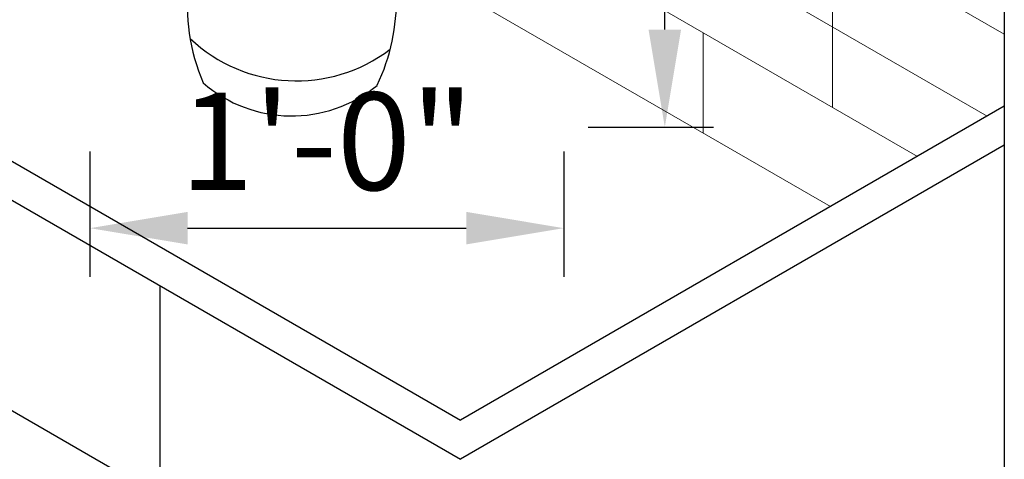
# Model space of a CAD drawing. Units: inches. Extents: x 5770 to 11891, y 3254 to 6808.
# Tile 9 of 15: x 6048 to 6073, y 3403 to 3414. Entities that reach past the tile are written whole.
import ezdxf

# ---------------------------------------------------------------- set-up
doc = ezdxf.new("R2010")
doc.units = ezdxf.units.IN
for name, color, linetype, lineweight in [('A-ANNO-DIMS', 2, 'Continuous', 18), ('A-DOOR', 4, 'Continuous', 25), ('A-FURN', 8, 'Continuous', 25), ('A-WALL-PATT', 8, 'Continuous', 13)]:
    doc.layers.add(name, color=color, linetype=linetype, lineweight=lineweight)
doc.styles.get("Standard").update_dxf_attribs({"font": 'arial.ttf'})
doc.dimstyles.new('ISO-25', dxfattribs={"dimtxt": 2.5, "dimasz": 2.5, "dimexe": 1.25, "dimexo": 0.625, "dimtad": 1, "dimdec": 0, "dimlunit": 3, "dimtxsty": 'Standard', "dimcen": 2.5, "dimadec": 0, "dimazin": 0, "dimtfac": 1, "dimtdec": 0, "dimtmove": 0, "dimatfit": 3, "dimfxl": 1, "dimarcsym": 0})

# ---------------------------------------------------------------- blocks, each defined once
blk = doc.blocks.new('POT TREE')
for centre, radius, start, end in [((6057.241, 3414.341), 4.914, 142.3065, 203.4115), ((6052.61, 3414.509), 5.072, 334.4796, 28.1737), ((6055.12, 3416.4), 3.962, 226.5306, 307.3215), ((6054.997, 3414.987), 3.448, 228.9077, 309.4208)]:
    blk.add_arc(centre, radius, start, end)
blk.add_ellipse((6055.216, 3417.125), major_axis=(-1.864, 0.221), ratio=0.431649, start_param=4.964377, end_param=10.722247)
for points, knots in [([(6056.099, 3428.486), (6056.067, 3428.368), (6056.02, 3428.192), (6055.948, 3427.91), (6056.053, 3427.786), (6056.115, 3427.713)], [0, 0, 0, 0, 0.3734405, 0.5554394, 0.8239698, 0.8239698, 0.8239698, 0.8239698]), ([(6056.207, 3427.847), (6056.213, 3427.924), (6056.224, 3428.053), (6056.232, 3428.215), (6056.298, 3428.293), (6056.297, 3428.355), (6056.343, 3428.437), (6056.403, 3428.481), (6056.451, 3428.516)], [0, 0, 0, 0, 0.2339594, 0.3926456, 0.4649395, 0.5251746, 0.5691994, 0.7434006, 0.7434006, 0.7434006, 0.7434006]), ([(6055.216, 3417.125), (6055.336, 3418.48), (6055.487, 3420.181), (6056.331, 3422.342), (6055.715, 3423.715), (6056.354, 3425.55), (6055.582, 3427.539), (6056.504, 3428.093), (6056.597, 3428.149)], [0, 0, 0, 0, 4.080433, 5.124412, 6.755782, 8.14589, 10.974647, 11.292118, 11.292118, 11.292118, 11.292118]), ([(6056, 3427.411), (6055.979, 3427.477), (6055.946, 3427.582), (6055.946, 3427.752), (6055.806, 3427.869), (6055.784, 3428.034), (6055.784, 3428.159), (6055.766, 3428.202), (6055.759, 3428.218)], [0, 0, 0, 0, 0.2083526, 0.33199, 0.4828354, 0.7148467, 0.8018251, 0.8541407, 0.8541407, 0.8541407, 0.8541407]), ([(6056.371, 3428.002), (6056.422, 3428.039), (6056.532, 3428.118), (6056.727, 3428.199), (6056.886, 3428.139), (6056.964, 3428.199), (6056.961, 3428.223), (6056.96, 3428.232)], [0, 0, 0, 0, 0.1895566, 0.4093046, 0.6024508, 0.6414497, 0.6690189, 0.6690189, 0.6690189, 0.6690189]), ([(6055.967, 3426.585), (6055.915, 3426.698), (6055.838, 3426.866), (6055.755, 3427.096), (6055.662, 3427.248), (6055.479, 3427.316), (6055.344, 3427.566), (6055.436, 3427.759), (6055.492, 3427.874)], [0, 0, 0, 0, 0.371816, 0.552306, 0.74044, 0.877889, 1.120726, 1.482251, 1.482251, 1.482251, 1.482251]), ([(6056.064, 3427.611), (6056.145, 3427.655), (6056.269, 3427.724), (6056.427, 3427.889), (6056.588, 3427.869), (6056.72, 3427.903), (6056.741, 3427.953), (6056.749, 3427.972)], [0, 0, 0, 0, 0.2777951, 0.4294687, 0.6442569, 0.739735, 0.8005553, 0.8005553, 0.8005553, 0.8005553]), ([(6059.539, 3427.305), (6059.549, 3427.361), (6059.566, 3427.456), (6059.622, 3427.589), (6059.57, 3427.693), (6059.584, 3427.781), (6059.582, 3427.83), (6059.582, 3427.851)], [0, 0, 0, 0, 0.170284, 0.2915753, 0.4095788, 0.4920381, 0.5552227, 0.5552227, 0.5552227, 0.5552227]), ([(6055.746, 3427.727), (6055.745, 3427.704), (6055.742, 3427.656), (6055.802, 3427.595), (6055.813, 3427.51), (6055.793, 3427.397), (6055.923, 3427.324), (6055.949, 3427.228), (6055.963, 3427.179)], [0, 0, 0, 0, 0.0663677, 0.1385674, 0.2396579, 0.315315, 0.459478, 0.6088633, 0.6088633, 0.6088633, 0.6088633]), ([(6055.99, 3427.367), (6056.038, 3427.373), (6056.112, 3427.383), (6056.172, 3427.461), (6056.237, 3427.541), (6056.366, 3427.57), (6056.481, 3427.602), (6056.575, 3427.618), (6056.602, 3427.667), (6056.64, 3427.68), (6056.661, 3427.712), (6056.683, 3427.71), (6056.69, 3427.709)], [0, 0, 0, 0, 0.1365482, 0.2128619, 0.286554, 0.4402885, 0.5819688, 0.663825, 0.70336, 0.7384662, 0.7808805, 0.8013382, 0.8013382, 0.8013382, 0.8013382]), ([(6059.29, 3426.939), (6059.259, 3427.006), (6059.196, 3427.136), (6059.318, 3427.315), (6059.332, 3427.522), (6059.269, 3427.641), (6059.235, 3427.705)], [0, 0, 0, 0, 0.2050478, 0.4040971, 0.5914015, 0.8021175, 0.8021175, 0.8021175, 0.8021175]), ([(6059.29, 3426.939), (6059.343, 3427.011), (6059.426, 3427.125), (6059.515, 3427.313), (6059.674, 3427.364), (6059.891, 3427.379), (6059.816, 3427.58), (6059.884, 3427.567), (6059.904, 3427.563)], [0, 0, 0, 0, 0.2714027, 0.4305119, 0.5814667, 0.7785807, 0.9004742, 0.951926, 0.951926, 0.951926, 0.951926]), ([(6056.605, 3427.524), (6056.509, 3427.444), (6056.38, 3427.336), (6056.327, 3427.13), (6056.226, 3427.052), (6056.128, 3427.019), (6056.036, 3426.975), (6056.021, 3426.89), (6055.939, 3426.905), (6055.963, 3426.892), (6055.973, 3426.886)], [0, 0, 0, 0, 0.3596279, 0.4887998, 0.612961, 0.7210682, 0.8063572, 0.9000005, 0.9307269, 0.9560982, 0.9560982, 0.9560982, 0.9560982]), ([(6055.977, 3426.474), (6055.99, 3426.502), (6056.028, 3426.582), (6056.121, 3426.639), (6056.2, 3426.712), (6056.242, 3426.835), (6056.362, 3426.959), (6056.525, 3427.032), (6056.66, 3427.104), (6056.792, 3427.159), (6056.821, 3427.278), (6056.814, 3427.378), (6056.873, 3427.411), (6056.899, 3427.426)], [0, 0, 0, 0, 0.092214, 0.262657, 0.315664, 0.410651, 0.642816, 0.809137, 0.941877, 1.112577, 1.190652, 1.298465, 1.380948, 1.380948, 1.380948, 1.380948]), ([(6056.095, 3422.726), (6056.606, 3423.324), (6057.847, 3424.774), (6058.906, 3426.363), (6059.529, 3427.297)], [0, 0, 0, 0, 2.356363, 5.722003, 5.722003, 5.722003, 5.722003]), ([(6056.056, 3425.848), (6056.006, 3425.989), (6055.924, 3426.218), (6055.821, 3426.517), (6055.761, 3426.712), (6055.708, 3426.876), (6055.625, 3426.962), (6055.572, 3427.054), (6055.493, 3427.115), (6055.42, 3427.147), (6055.376, 3427.166)], [0, 0, 0, 0, 0.450624, 0.730149, 0.944944, 1.068285, 1.240151, 1.294175, 1.386296, 1.531529, 1.531529, 1.531529, 1.531529]), ([(6058.831, 3426.258), (6058.841, 3426.314), (6058.865, 3426.442), (6058.859, 3426.622), (6058.864, 3426.782), (6058.891, 3426.906), (6058.89, 3427.037), (6058.917, 3427.145), (6058.938, 3427.235), (6058.962, 3427.266), (6058.975, 3427.282)], [0, 0, 0, 0, 0.170516, 0.389854, 0.537702, 0.648645, 0.771235, 0.925907, 0.983276, 1.044113, 1.044113, 1.044113, 1.044113]), ([(6059.29, 3426.939), (6059.328, 3426.955), (6059.413, 3426.99), (6059.547, 3427.012), (6059.733, 3427.027), (6059.904, 3427.081), (6060.076, 3427.185), (6060.184, 3427.182), (6060.249, 3427.18)], [0, 0, 0, 0, 0.1235803, 0.275185, 0.4036544, 0.6827396, 0.8054315, 0.9964413, 0.9964413, 0.9964413, 0.9964413]), ([(6056.054, 3424.972), (6055.977, 3425.109), (6055.832, 3425.363), (6055.757, 3425.794), (6055.716, 3426.157), (6055.592, 3426.405), (6055.526, 3426.622), (6055.441, 3426.739), (6055.385, 3426.816)], [0, 0, 0, 0, 0.467532, 0.868461, 1.30425, 1.550258, 1.694478, 1.979135, 1.979135, 1.979135, 1.979135]), ([(6056.377, 3426.818), (6056.352, 3426.755), (6056.308, 3426.64), (6056.245, 3426.496), (6056.206, 3426.387), (6056.142, 3426.323), (6056.096, 3426.241), (6056.077, 3426.145), (6056.033, 3426.102), (6056.017, 3426.086)], [0, 0, 0, 0, 0.2037441, 0.3695408, 0.4757745, 0.5419956, 0.6389372, 0.7550592, 0.8219377, 0.8219377, 0.8219377, 0.8219377]), ([(6056.056, 3425.848), (6056.123, 3425.96), (6056.303, 3426.262), (6056.779, 3426.349), (6056.935, 3426.684), (6056.925, 3426.814), (6056.92, 3426.871)], [0, 0, 0, 0, 0.381595, 1.02877, 1.247836, 1.417617, 1.417617, 1.417617, 1.417617]), ([(6058.261, 3425.438), (6058.291, 3425.526), (6058.343, 3425.679), (6058.339, 3425.9), (6058.37, 3426.087), (6058.319, 3426.305), (6058.353, 3426.513), (6058.32, 3426.678), (6058.317, 3426.794), (6058.344, 3426.858), (6058.363, 3426.902)], [0, 0, 0, 0, 0.275722, 0.478551, 0.660336, 0.838715, 1.138147, 1.278337, 1.3416, 1.482993, 1.482993, 1.482993, 1.482993]), ([(6058.563, 3425.867), (6058.56, 3426.061), (6058.555, 3426.39), (6058.4, 3426.795), (6058.513, 3426.977), (6058.549, 3427.032), (6058.551, 3427.035)], [0, 0, 0, 0, 0.586596, 0.998805, 1.183674, 1.195699, 1.195699, 1.195699, 1.195699]), ([(6058.962, 3426.451), (6059.049, 3426.488), (6059.206, 3426.554), (6059.435, 3426.627), (6059.634, 3426.652), (6059.81, 3426.698), (6059.948, 3426.696), (6060.018, 3426.762), (6060.066, 3426.814), (6060.121, 3426.838), (6060.156, 3426.854)], [0, 0, 0, 0, 0.283693, 0.509561, 0.721223, 0.878225, 1.064501, 1.097071, 1.163997, 1.27537, 1.27537, 1.27537, 1.27537]), ([(6059.16, 3426.744), (6059.203, 3426.742), (6059.314, 3426.736), (6059.465, 3426.81), (6059.623, 3426.872), (6059.755, 3426.911), (6059.886, 3426.903), (6059.993, 3426.931), (6060.073, 3426.99), (6060.123, 3427.004), (6060.148, 3427.011)], [0, 0, 0, 0, 0.127889, 0.331448, 0.488133, 0.640962, 0.738356, 0.878783, 0.95994, 1.034357, 1.034357, 1.034357, 1.034357]), ([(6055.951, 3424.314), (6055.922, 3424.36), (6055.81, 3424.54), (6055.651, 3424.735), (6055.521, 3424.997), (6055.443, 3425.215), (6055.337, 3425.488), (6054.988, 3425.625), (6055.168, 3425.925), (6055.049, 3426.109), (6054.991, 3426.355), (6054.968, 3426.555), (6054.951, 3426.702)], [0, 0, 0, 0, 0.163711, 0.635891, 0.747378, 1.038356, 1.335228, 1.608013, 1.929766, 2.083186, 2.238732, 2.684923, 2.684923, 2.684923, 2.684923]), ([(6057.656, 3424.618), (6057.652, 3424.844), (6057.647, 3425.111), (6057.61, 3425.475), (6057.704, 3425.744), (6057.631, 3426.115), (6057.55, 3426.461), (6057.608, 3426.662), (6057.627, 3426.731)], [0, 0, 0, 0, 0.681083, 0.80233, 1.088716, 1.507668, 1.913958, 2.127718, 2.127718, 2.127718, 2.127718]), ([(6057.812, 3424.824), (6057.859, 3424.939), (6057.966, 3425.201), (6057.98, 3425.575), (6057.986, 3425.877), (6058.063, 3426.137), (6057.992, 3426.354), (6057.93, 3426.581), (6057.997, 3426.635), (6058.014, 3426.65)], [0, 0, 0, 0, 0.369909, 0.844557, 1.104784, 1.280935, 1.632037, 1.811788, 1.877667, 1.877667, 1.877667, 1.877667]), ([(6056.072, 3425.293), (6056.133, 3425.505), (6056.266, 3425.967), (6056.936, 3426.129), (6056.94, 3426.432), (6056.94, 3426.477)], [0, 0, 0, 0, 0.63578, 1.387331, 1.51754, 1.51754, 1.51754, 1.51754]), ([(6057.341, 3423.955), (6057.366, 3424.231), (6057.406, 3424.685), (6057.283, 3425.234), (6057.35, 3425.634), (6057.475, 3425.987), (6057.255, 3426.274), (6057.321, 3426.442), (6057.341, 3426.491)], [0, 0, 0, 0, 0.827857, 1.361014, 1.650618, 2.046768, 2.412651, 2.567148, 2.567148, 2.567148, 2.567148]), ([(6058.777, 3426.179), (6058.935, 3426.238), (6059.178, 3426.33), (6059.474, 3426.418), (6059.645, 3426.392), (6059.742, 3426.437), (6059.823, 3426.499), (6059.909, 3426.479), (6059.995, 3426.5), (6060.058, 3426.496), (6060.091, 3426.519), (6060.093, 3426.521)], [0, 0, 0, 0, 0.507912, 0.783706, 0.910821, 1.010253, 1.096153, 1.201661, 1.253677, 1.364003, 1.37374, 1.37374, 1.37374, 1.37374]), ([(6056.038, 3424.843), (6056.072, 3424.898), (6056.124, 3424.984), (6056.15, 3425.124), (6056.224, 3425.253), (6056.367, 3425.285), (6056.418, 3425.409), (6056.447, 3425.536), (6056.633, 3425.585), (6056.578, 3425.765), (6056.728, 3425.791), (6056.822, 3425.814), (6056.921, 3425.958), (6057.035, 3426.009), (6057.139, 3426.056)], [0, 0, 0, 0, 0.192002, 0.297038, 0.424323, 0.617299, 0.671515, 0.818658, 0.985168, 1.116162, 1.215874, 1.36714, 1.40004, 1.729093, 1.729093, 1.729093, 1.729093]), ([(6058.635, 3425.972), (6058.738, 3426.004), (6058.893, 3426.052), (6059.061, 3426.159), (6059.218, 3426.171), (6059.334, 3426.132), (6059.411, 3426.181), (6059.424, 3426.213), (6059.433, 3426.237), (6059.438, 3426.25)], [0, 0, 0, 0, 0.3205478, 0.4875046, 0.5825134, 0.7880727, 0.8113343, 0.8451959, 0.8888695, 0.8888695, 0.8888695, 0.8888695]), ([(6055.908, 3423.774), (6055.633, 3423.935), (6055.268, 3424.15), (6055.37, 3424.761), (6054.903, 3424.997), (6054.405, 3425.105), (6054.23, 3425.467), (6053.986, 3425.639), (6053.974, 3425.758), (6053.967, 3425.819)], [0, 0, 0, 0, 0.828493, 1.099501, 1.668133, 2.09953, 2.614238, 2.775429, 2.952527, 2.952527, 2.952527, 2.952527]), ([(6055.474, 3425.905), (6055.51, 3425.799), (6055.556, 3425.669), (6055.622, 3425.499), (6055.623, 3425.305), (6055.834, 3425.19), (6055.818, 3425.005), (6055.912, 3424.948), (6055.91, 3424.824), (6055.955, 3424.719), (6055.995, 3424.675), (6056.01, 3424.659)], [0, 0, 0, 0, 0.336378, 0.413394, 0.545538, 0.892702, 0.982578, 1.034981, 1.194475, 1.310114, 1.373927, 1.373927, 1.373927, 1.373927]), ([(6058.421, 3425.664), (6058.505, 3425.707), (6058.644, 3425.779), (6058.864, 3425.834), (6059.06, 3425.877), (6059.217, 3425.861), (6059.319, 3425.896), (6059.371, 3425.9), (6059.397, 3425.925), (6059.403, 3425.931)], [0, 0, 0, 0, 0.283751, 0.46616, 0.680012, 0.883292, 0.92268, 1.004792, 1.029716, 1.029716, 1.029716, 1.029716]), ([(6055.951, 3424.314), (6055.971, 3424.342), (6056.04, 3424.439), (6056.158, 3424.572), (6056.282, 3424.757), (6056.522, 3424.974), (6056.461, 3425.359), (6056.847, 3425.665), (6057.142, 3425.719), (6057.374, 3425.762)], [0, 0, 0, 0, 0.103537, 0.354957, 0.533042, 0.771117, 1.289622, 1.481323, 2.177692, 2.177692, 2.177692, 2.177692]), ([(6058.261, 3425.438), (6058.37, 3425.457), (6058.551, 3425.488), (6058.776, 3425.584), (6058.921, 3425.67), (6059.047, 3425.695), (6059.147, 3425.687), (6059.211, 3425.696), (6059.244, 3425.701)], [0, 0, 0, 0, 0.330364, 0.547312, 0.729955, 0.831797, 0.929171, 1.027126, 1.027126, 1.027126, 1.027126]), ([(6055.918, 3424.061), (6055.807, 3424.119), (6055.605, 3424.225), (6055.669, 3424.572), (6055.437, 3424.761), (6055.344, 3425.012), (6055.093, 3425.129), (6054.941, 3425.333), (6054.69, 3425.32), (6054.659, 3425.414), (6054.651, 3425.437)], [0, 0, 0, 0, 0.336493, 0.612709, 0.889575, 1.168065, 1.376144, 1.687858, 1.898629, 1.969205, 1.969205, 1.969205, 1.969205]), ([(6058.016, 3425.1), (6058.09, 3425.123), (6058.24, 3425.171), (6058.377, 3425.249), (6058.448, 3425.288)], [0, 0, 0, 0, 0.2298962, 0.4721725, 0.4721725, 0.4721725, 0.4721725]), ([(6058.448, 3425.288), (6058.521, 3425.33), (6058.626, 3425.39), (6058.771, 3425.413), (6058.839, 3425.441), (6058.89, 3425.468), (6059.001, 3425.522), (6059.117, 3425.5), (6059.209, 3425.483)], [0, 0, 0, 0, 0.2475713, 0.3610151, 0.4350864, 0.4658518, 0.5335827, 0.8019321, 0.8019321, 0.8019321, 0.8019321]), ([(6057.656, 3424.618), (6057.702, 3424.649), (6057.811, 3424.723), (6057.967, 3424.784), (6058.092, 3424.912), (6058.24, 3424.946), (6058.406, 3424.93), (6058.532, 3424.97), (6058.635, 3424.985), (6058.698, 3425.029), (6058.74, 3425.056), (6058.818, 3425.086), (6058.86, 3425.114), (6058.898, 3425.14)], [0, 0, 0, 0, 0.169056, 0.394003, 0.492513, 0.697087, 0.817485, 0.993544, 1.088828, 1.12295, 1.222592, 1.236685, 1.373008, 1.373008, 1.373008, 1.373008]), ([(6052.095, 3424.128), (6051.893, 3424.174), (6051.588, 3424.244), (6051.432, 3424.772), (6050.96, 3424.716), (6050.677, 3424.834), (6050.499, 3424.886), (6050.399, 3424.881), (6050.277, 3424.893), (6050.323, 3424.931), (6050.355, 3424.957)], [0, 0, 0, 0, 0.567769, 0.855404, 1.45352, 1.680633, 1.805502, 1.990259, 2.022667, 2.10403, 2.10403, 2.10403, 2.10403]), ([(6052.343, 3424.042), (6052.218, 3424.175), (6052.017, 3424.389), (6051.803, 3424.65), (6051.728, 3424.895), (6051.471, 3424.824), (6051.572, 3425.006), (6051.486, 3424.99), (6051.442, 3424.981)], [0, 0, 0, 0, 0.542059, 0.875538, 1.040909, 1.212562, 1.305796, 1.401779, 1.401779, 1.401779, 1.401779]), ([(6055.908, 3423.774), (6056.079, 3423.881), (6056.273, 3424.004), (6056.294, 3424.296), (6056.442, 3424.382), (6056.436, 3424.57), (6056.566, 3424.599), (6056.652, 3424.629), (6056.706, 3424.683), (6056.749, 3424.715), (6056.785, 3424.758), (6056.813, 3424.79), (6056.828, 3424.806)], [0, 0, 0, 0, 0.542154, 0.617715, 0.844166, 0.985871, 1.075503, 1.203366, 1.260039, 1.30062, 1.363236, 1.427954, 1.427954, 1.427954, 1.427954]), ([(6057.262, 3424.117), (6057.321, 3424.22), (6057.45, 3424.44), (6057.801, 3424.465), (6057.98, 3424.628), (6058.071, 3424.73), (6058.139, 3424.775), (6058.206, 3424.814), (6058.293, 3424.816), (6058.392, 3424.838), (6058.585, 3424.884), (6058.731, 3424.952), (6058.845, 3425.005)], [0, 0, 0, 0, 0.337635, 0.723781, 0.946218, 1.049759, 1.130989, 1.190526, 1.278087, 1.386469, 1.496256, 1.869563, 1.869563, 1.869563, 1.869563]), ([(6053.102, 3423.341), (6052.97, 3423.509), (6052.8, 3423.727), (6052.762, 3424.081), (6052.701, 3424.27), (6052.615, 3424.453), (6052.462, 3424.594), (6052.282, 3424.626), (6052.055, 3424.59), (6052.073, 3424.693), (6052.08, 3424.733)], [0, 0, 0, 0, 0.618637, 0.799298, 1.058478, 1.209073, 1.406969, 1.64005, 1.800082, 1.901705, 1.901705, 1.901705, 1.901705]), ([(6059.336, 3423.893), (6059.408, 3424.012), (6059.539, 3424.232), (6059.834, 3424.307), (6059.954, 3424.433), (6059.99, 3424.55), (6060.142, 3424.55), (6060.219, 3424.694), (6060.331, 3424.733), (6060.401, 3424.761), (6060.419, 3424.769)], [0, 0, 0, 0, 0.400751, 0.736445, 0.858272, 0.903351, 1.088652, 1.199604, 1.364928, 1.425221, 1.425221, 1.425221, 1.425221]), ([(6060.005, 3424.184), (6060.12, 3424.224), (6060.289, 3424.284), (6060.491, 3424.373), (6060.647, 3424.398), (6060.679, 3424.537), (6060.828, 3424.549), (6060.995, 3424.593), (6061.2, 3424.559), (6061.253, 3424.642), (6061.255, 3424.646)], [0, 0, 0, 0, 0.362377, 0.533627, 0.680662, 0.781131, 0.894461, 1.071848, 1.350792, 1.364242, 1.364242, 1.364242, 1.364242]), ([(6051.253, 3424.176), (6051.125, 3424.167), (6050.939, 3424.154), (6050.737, 3424.369), (6050.418, 3424.319), (6050.137, 3424.329), (6049.924, 3424.328), (6049.85, 3424.328), (6049.829, 3424.328)], [0, 0, 0, 0, 0.359068, 0.523067, 0.822385, 1.235556, 1.394449, 1.458006, 1.458006, 1.458006, 1.458006]), ([(6055.646, 3420.285), (6054.953, 3420.935), (6053.781, 3422.034), (6052.605, 3424.433), (6051.084, 3424.175), (6050.302, 3424.043)], [0, 0, 0, 0, 2.90941, 4.916012, 7.044236, 7.044236, 7.044236, 7.044236]), ([(6053.304, 3423.041), (6053.281, 3423.107), (6053.242, 3423.221), (6053.213, 3423.38), (6053.212, 3423.562), (6053.093, 3423.731), (6053.031, 3423.964), (6053.134, 3424.1), (6053.132, 3424.22), (6053.101, 3424.267), (6053.085, 3424.294)], [0, 0, 0, 0, 0.211774, 0.357994, 0.485633, 0.747154, 0.967772, 1.145664, 1.219006, 1.311906, 1.311906, 1.311906, 1.311906]), ([(6054.095, 3421.885), (6053.944, 3422.23), (6053.77, 3422.627), (6053.839, 3423.155), (6053.889, 3423.378), (6053.801, 3423.541), (6053.791, 3423.682), (6053.725, 3423.875), (6053.744, 3424.161), (6053.726, 3424.363), (6053.717, 3424.466)], [0, 0, 0, 0, 1.080878, 1.246414, 1.604364, 1.717568, 1.785951, 2.023042, 2.322993, 2.633061, 2.633061, 2.633061, 2.633061]), ([(6055.914, 3421.233), (6056.513, 3421.466), (6057.612, 3421.896), (6058.722, 3423.014), (6059.604, 3424.466), (6060.6, 3424.086), (6061.117, 3423.89)], [0, 0, 0, 0, 1.890611, 3.471497, 4.822432, 6.275175, 6.275175, 6.275175, 6.275175]), ([(6055.918, 3424.061), (6055.945, 3424.099), (6055.999, 3424.179), (6056.084, 3424.275), (6056.149, 3424.349), (6056.161, 3424.4), (6056.174, 3424.429), (6056.192, 3424.458), (6056.228, 3424.464), (6056.232, 3424.481), (6056.233, 3424.483)], [0, 0, 0, 0, 0.1386217, 0.290258, 0.3867591, 0.4253621, 0.4453978, 0.4816222, 0.5256508, 0.5320801, 0.5320801, 0.5320801, 0.5320801]), ([(6058.834, 3423.265), (6058.889, 3423.458), (6058.95, 3423.672), (6059.018, 3423.985), (6059.186, 3424.087), (6059.322, 3424.218), (6059.346, 3424.318), (6059.405, 3424.426), (6059.518, 3424.378), (6059.62, 3424.335)], [0, 0, 0, 0, 0.604353, 0.674045, 0.943845, 1.144991, 1.220534, 1.250613, 1.50171, 1.50171, 1.50171, 1.50171]), ([(6060.567, 3424.085), (6060.678, 3424.128), (6060.816, 3424.182), (6061.002, 3424.203), (6061.101, 3424.216), (6061.239, 3424.21), (6061.349, 3424.271), (6061.436, 3424.34), (6061.493, 3424.355), (6061.553, 3424.359), (6061.641, 3424.368), (6061.774, 3424.381), (6061.846, 3424.524), (6061.933, 3424.51), (6061.969, 3424.504)], [0, 0, 0, 0, 0.353763, 0.440342, 0.560317, 0.653707, 0.850793, 0.918069, 0.984218, 1.021734, 1.10046, 1.251722, 1.394315, 1.495093, 1.495093, 1.495093, 1.495093]), ([(6052.439, 3423.994), (6052.37, 3424.027), (6052.226, 3424.095), (6052.118, 3423.882), (6051.811, 3423.894), (6051.509, 3423.998), (6051.113, 3423.84), (6050.808, 3423.8), (6050.45, 3423.729), (6050.195, 3423.714), (6050.053, 3423.795), (6050.042, 3423.802)], [0, 0, 0, 0, 0.199212, 0.412008, 0.540446, 1.07049, 1.336159, 1.784437, 1.991377, 2.444385, 2.482266, 2.482266, 2.482266, 2.482266]), ([(6053.883, 3422.424), (6053.784, 3422.656), (6053.655, 3422.959), (6053.263, 3423.297), (6053.425, 3423.67), (6053.49, 3424.036), (6053.35, 3424.195), (6053.295, 3424.258)], [0, 0, 0, 0, 0.757434, 0.989726, 1.429851, 1.797091, 2.0391, 2.0391, 2.0391, 2.0391]), ([(6058.308, 3422.628), (6058.351, 3422.73), (6058.434, 3422.922), (6058.496, 3423.192), (6058.488, 3423.425), (6058.594, 3423.581), (6058.644, 3423.82), (6058.789, 3424.077), (6058.991, 3424.16), (6059.071, 3424.193)], [0, 0, 0, 0, 0.330054, 0.62708, 0.829768, 1.006692, 1.17071, 1.565043, 1.817324, 1.817324, 1.817324, 1.817324]), ([(6059.433, 3424.046), (6059.6, 3424.055), (6059.869, 3424.069), (6060.149, 3423.884), (6060.339, 3423.83), (6060.478, 3423.858), (6060.542, 3423.827), (6060.583, 3423.807)], [0, 0, 0, 0, 0.485239, 0.777831, 0.986173, 1.058443, 1.191294, 1.191294, 1.191294, 1.191294]), ([(6060.404, 3424.13), (6060.481, 3424.077), (6060.651, 3423.96), (6060.992, 3423.771), (6061.203, 3423.563), (6061.333, 3423.435)], [0, 0, 0, 0, 0.279864, 0.61954, 1.163685, 1.163685, 1.163685, 1.163685]), ([(6061.117, 3423.89), (6061.136, 3423.871), (6061.182, 3423.827), (6061.296, 3423.775), (6061.44, 3423.829), (6061.624, 3423.787), (6061.743, 3423.735), (6061.814, 3423.705)], [0, 0, 0, 0, 0.0805276, 0.1908805, 0.3539186, 0.511807, 0.7436297, 0.7436297, 0.7436297, 0.7436297]), ([(6052.99, 3423.487), (6052.815, 3423.575), (6052.516, 3423.724), (6052.091, 3423.65), (6051.784, 3423.611), (6051.538, 3423.669), (6051.349, 3423.573), (6051.175, 3423.596), (6051.077, 3423.631), (6051.031, 3423.647)], [0, 0, 0, 0, 0.568997, 0.970672, 1.257313, 1.499172, 1.696498, 1.862231, 2.008965, 2.008965, 2.008965, 2.008965]), ([(6053.128, 3423.304), (6052.945, 3423.442), (6052.696, 3423.63), (6052.359, 3423.482), (6052.123, 3423.424), (6051.892, 3423.426), (6051.639, 3423.459), (6051.442, 3423.491), (6051.286, 3423.441), (6051.178, 3423.384), (6051.122, 3423.496), (6051.062, 3423.486), (6051.038, 3423.481)], [0, 0, 0, 0, 0.612219, 0.830799, 1.053962, 1.343292, 1.51324, 1.82687, 1.906932, 2.021983, 2.121771, 2.190079, 2.190079, 2.190079, 2.190079]), ([(6057.366, 3421.886), (6057.481, 3422.012), (6057.623, 3422.17), (6057.727, 3422.4), (6057.798, 3422.472), (6057.863, 3422.574), (6057.878, 3422.763), (6057.949, 3422.994), (6057.791, 3423.308), (6058.079, 3423.393), (6058.156, 3423.515), (6058.186, 3423.561)], [0, 0, 0, 0, 0.507365, 0.630934, 0.750401, 0.807356, 0.99106, 1.298058, 1.54708, 1.813675, 1.980924, 1.980924, 1.980924, 1.980924]), ([(6059.095, 3423.618), (6059.188, 3423.647), (6059.316, 3423.688), (6059.486, 3423.699), (6059.611, 3423.72), (6059.774, 3423.648), (6059.944, 3423.627), (6060.099, 3423.632), (6060.195, 3423.604), (6060.255, 3423.589), (6060.284, 3423.582)], [0, 0, 0, 0, 0.290651, 0.399486, 0.511705, 0.662964, 0.915828, 1.024132, 1.123744, 1.212466, 1.212466, 1.212466, 1.212466]), ([(6057.012, 3421.697), (6057.043, 3421.847), (6057.134, 3422.295), (6057.798, 3422.701), (6057.549, 3423.097), (6057.468, 3423.242), (6057.473, 3423.338), (6057.475, 3423.369)], [0, 0, 0, 0, 0.465095, 1.381617, 1.582999, 1.778125, 1.868177, 1.868177, 1.868177, 1.868177]), ([(6058.747, 3423.147), (6058.871, 3423.174), (6059.088, 3423.221), (6059.303, 3423.434), (6059.548, 3423.398), (6059.734, 3423.43), (6059.881, 3423.375), (6059.944, 3423.354), (6059.967, 3423.347)], [0, 0, 0, 0, 0.377467, 0.661703, 0.822215, 1.087282, 1.215987, 1.286799, 1.286799, 1.286799, 1.286799]), ([(6053.386, 3422.911), (6053.319, 3422.965), (6053.196, 3423.066), (6052.997, 3423.089), (6052.887, 3423.18), (6052.784, 3423.172), (6052.672, 3423.146), (6052.482, 3423.153), (6052.305, 3423.116), (6052.168, 3423.234), (6052.112, 3423.113), (6052.076, 3423.184), (6052.058, 3423.22)], [0, 0, 0, 0, 0.2532, 0.467362, 0.579011, 0.658111, 0.76336, 0.926661, 1.225585, 1.285316, 1.367609, 1.455256, 1.455256, 1.455256, 1.455256]), ([(6057.782, 3422.159), (6057.848, 3422.194), (6057.948, 3422.247), (6057.983, 3422.484), (6058.115, 3422.666), (6058.083, 3422.874), (6058.11, 3422.976), (6058.129, 3423.052), (6058.148, 3423.095), (6058.156, 3423.114)], [0, 0, 0, 0, 0.206446, 0.312525, 0.690412, 0.832163, 0.923619, 1.005094, 1.065366, 1.065366, 1.065366, 1.065366]), ([(6058.442, 3422.774), (6058.529, 3422.832), (6058.661, 3422.92), (6058.919, 3423.02), (6059.139, 3422.965), (6059.366, 3422.954), (6059.496, 3422.989), (6059.612, 3422.989), (6059.663, 3423.038), (6059.737, 3423.066), (6059.786, 3423.066), (6059.817, 3423.066)], [0, 0, 0, 0, 0.314833, 0.47653, 0.809502, 0.966328, 1.154795, 1.214977, 1.302026, 1.35401, 1.447623, 1.447623, 1.447623, 1.447623]), ([(6053.514, 3422.708), (6053.439, 3422.751), (6053.333, 3422.813), (6053.158, 3422.904), (6053.015, 3422.892), (6052.87, 3422.865), (6052.704, 3422.836), (6052.574, 3422.924), (6052.436, 3422.96), (6052.327, 3422.917), (6052.207, 3422.881), (6052.131, 3422.931), (6052.115, 3422.96), (6052.105, 3422.978)], [0, 0, 0, 0, 0.261711, 0.370131, 0.582712, 0.66806, 0.81934, 1.066406, 1.111973, 1.240926, 1.409664, 1.445312, 1.505627, 1.505627, 1.505627, 1.505627]), ([(6053.711, 3422.403), (6053.634, 3422.436), (6053.477, 3422.502), (6053.266, 3422.504), (6053.133, 3422.505), (6053.046, 3422.504), (6052.964, 3422.514), (6052.871, 3422.48), (6052.791, 3422.486), (6052.715, 3422.486), (6052.602, 3422.477), (6052.532, 3422.566), (6052.333, 3422.563), (6052.195, 3422.552), (6052.061, 3422.542)], [0, 0, 0, 0, 0.248192, 0.507613, 0.621751, 0.648397, 0.770142, 0.863413, 0.939511, 1.008, 1.091792, 1.268763, 1.280175, 1.684599, 1.684599, 1.684599, 1.684599]), ([(6058.106, 3422.43), (6058.148, 3422.451), (6058.241, 3422.497), (6058.39, 3422.448), (6058.529, 3422.477), (6058.674, 3422.492), (6058.804, 3422.517), (6058.927, 3422.547), (6058.989, 3422.56), (6059.04, 3422.564), (6059.031, 3422.619), (6059.053, 3422.65), (6059.07, 3422.674)], [0, 0, 0, 0, 0.136191, 0.301111, 0.440041, 0.556702, 0.739007, 0.8386, 0.929419, 0.944819, 0.971199, 1.059876, 1.059876, 1.059876, 1.059876]), ([(6054.055, 3421.936), (6053.704, 3422.141), (6053.282, 3422.388), (6052.829, 3422.079), (6052.591, 3421.952), (6052.296, 3421.974), (6052.122, 3421.985), (6052.023, 3421.991)], [0, 0, 0, 0, 1.043584, 1.256005, 1.602855, 1.825433, 2.126041, 2.126041, 2.126041, 2.126041]), ([(6057.679, 3422.086), (6057.809, 3422.103), (6058.076, 3422.14), (6058.365, 3422.152), (6058.546, 3422.197), (6058.621, 3422.188), (6058.735, 3422.179), (6058.839, 3422.21), (6058.968, 3422.217), (6059.07, 3422.14), (6059.222, 3422.147), (6059.333, 3422.22), (6059.355, 3422.359), (6059.421, 3422.328), (6059.447, 3422.316)], [0, 0, 0, 0, 0.393084, 0.806547, 0.867321, 0.945801, 1.031735, 1.209105, 1.268822, 1.409537, 1.566345, 1.691075, 1.797982, 1.871323, 1.871323, 1.871323, 1.871323]), ([(6057.214, 3421.8), (6057.318, 3421.831), (6057.489, 3421.882), (6057.767, 3421.934), (6058.014, 3421.911), (6058.239, 3421.862), (6058.413, 3421.88), (6058.536, 3421.902), (6058.624, 3421.948), (6058.698, 3421.994), (6058.799, 3421.986), (6058.862, 3422.016), (6058.895, 3422.032)], [0, 0, 0, 0, 0.325945, 0.533976, 0.844352, 1.062897, 1.220077, 1.365852, 1.432613, 1.519427, 1.617117, 1.724591, 1.724591, 1.724591, 1.724591]), ([(6057.012, 3421.697), (6057.294, 3421.68), (6057.596, 3421.661), (6057.945, 3421.695), (6058.029, 3421.623), (6058.155, 3421.652), (6058.353, 3421.615), (6058.438, 3421.764), (6058.496, 3421.868)], [0, 0, 0, 0, 0.853157, 0.913238, 1.027604, 1.147747, 1.282906, 1.590947, 1.590947, 1.590947, 1.590947]), ([(6058.416, 3420.323), (6058.386, 3420.43), (6058.328, 3420.635), (6058.378, 3420.941), (6058.35, 3421.253), (6058.588, 3421.407), (6058.557, 3421.519), (6058.552, 3421.536)], [0, 0, 0, 0, 0.328571, 0.626938, 0.928595, 1.215628, 1.267031, 1.267031, 1.267031, 1.267031]), ([(6058.53, 3420.428), (6058.572, 3420.547), (6058.639, 3420.74), (6058.526, 3420.984), (6058.558, 3421.16), (6058.632, 3421.286), (6058.65, 3421.419), (6058.678, 3421.511), (6058.692, 3421.555)], [0, 0, 0, 0, 0.358902, 0.587337, 0.76495, 0.869476, 1.023512, 1.159883, 1.159883, 1.159883, 1.159883]), ([(6058.778, 3420.669), (6058.794, 3420.753), (6058.823, 3420.909), (6058.77, 3421.086), (6058.703, 3421.247), (6058.802, 3421.3), (6058.856, 3421.388), (6058.849, 3421.477), (6058.842, 3421.531), (6058.841, 3421.54)], [0, 0, 0, 0, 0.2483439, 0.4590321, 0.5916982, 0.6641726, 0.7593593, 0.8908118, 0.9202375, 0.9202375, 0.9202375, 0.9202375]), ([(6058.975, 3420.87), (6058.978, 3420.953), (6058.984, 3421.082), (6058.943, 3421.261), (6059.065, 3421.361), (6059.083, 3421.483), (6059.082, 3421.566), (6059.082, 3421.58)], [0, 0, 0, 0, 0.2582523, 0.3969468, 0.4904461, 0.695008, 0.7388085, 0.7388085, 0.7388085, 0.7388085]), ([(6059.152, 3421.054), (6059.201, 3421.128), (6059.284, 3421.251), (6059.266, 3421.418), (6059.263, 3421.506), (6059.255, 3421.546), (6059.26, 3421.568), (6059.261, 3421.577)], [0, 0, 0, 0, 0.257058, 0.428605, 0.4834756, 0.5237874, 0.549599, 0.549599, 0.549599, 0.549599]), ([(6059.343, 3421.256), (6059.341, 3421.284), (6059.335, 3421.38), (6059.457, 3421.47), (6059.583, 3421.506), (6059.601, 3421.56), (6059.608, 3421.58)], [0, 0, 0, 0, 0.0794153, 0.2808618, 0.3854818, 0.4459081, 0.4459081, 0.4459081, 0.4459081]), ([(6052.739, 3420.786), (6052.7, 3420.865), (6052.63, 3421.006), (6052.541, 3421.199), (6052.517, 3421.351), (6052.45, 3421.424), (6052.432, 3421.46), (6052.424, 3421.478)], [0, 0, 0, 0, 0.2642834, 0.4700989, 0.6421411, 0.7030564, 0.762993, 0.762993, 0.762993, 0.762993]), ([(6053.044, 3420.562), (6053.066, 3420.709), (6053.095, 3420.908), (6052.951, 3421.137), (6052.889, 3421.29), (6052.893, 3421.412), (6052.878, 3421.454), (6052.875, 3421.462)], [0, 0, 0, 0, 0.4211546, 0.57187, 0.7991017, 0.9053512, 0.9310241, 0.9310241, 0.9310241, 0.9310241]), ([(6052.998, 3421.383), (6053.069, 3421.231), (6053.178, 3420.996), (6053.167, 3420.646), (6053.315, 3420.473), (6053.292, 3420.385)], [0, 0, 0, 0, 0.491062, 0.760416, 1.043151, 1.043151, 1.043151, 1.043151]), ([(6053.773, 3420.059), (6053.687, 3420.202), (6053.539, 3420.45), (6053.57, 3420.809), (6053.47, 3421.04), (6053.464, 3421.185), (6053.334, 3421.344), (6053.345, 3421.18), (6053.354, 3421.06)], [0, 0, 0, 0, 0.486789, 0.841844, 1.040934, 1.218264, 1.298858, 1.518651, 1.518651, 1.518651, 1.518651]), ([(6055.216, 3417.125), (6055.482, 3417.339), (6055.887, 3417.665), (6055.786, 3418.448), (6056.191, 3419.123), (6057.73, 3419.549), (6058.63, 3420.501), (6059.343, 3421.256)], [0, 0, 0, 0, 0.930345, 1.419949, 2.238038, 3.028538, 6.05988, 6.05988, 6.05988, 6.05988]), ([(6057.456, 3420.669), (6057.458, 3420.714), (6057.461, 3420.828), (6057.468, 3420.993), (6057.61, 3421.098), (6057.54, 3421.196), (6057.581, 3421.234), (6057.602, 3421.252)], [0, 0, 0, 0, 0.1343407, 0.3452256, 0.4766174, 0.5519158, 0.6245951, 0.6245951, 0.6245951, 0.6245951]), ([(6057.797, 3419.822), (6057.895, 3419.97), (6058.058, 3420.217), (6058.023, 3420.591), (6058.021, 3420.906), (6058.085, 3421.155), (6057.983, 3421.342), (6058.015, 3421.409), (6058.029, 3421.438)], [0, 0, 0, 0, 0.513113, 0.856104, 1.090795, 1.466282, 1.586294, 1.677635, 1.677635, 1.677635, 1.677635]), ([(6058.154, 3420.095), (6058.158, 3420.159), (6058.172, 3420.346), (6058.103, 3420.595), (6058.127, 3420.94), (6058.062, 3421.219), (6058.171, 3421.378), (6058.187, 3421.402)], [0, 0, 0, 0, 0.19319, 0.561329, 0.753109, 1.237908, 1.324083, 1.324083, 1.324083, 1.324083]), ([(6059.152, 3421.054), (6059.233, 3421.084), (6059.395, 3421.143), (6059.621, 3421.157), (6059.682, 3421.28), (6059.806, 3421.307), (6059.894, 3421.354), (6059.962, 3421.391)], [0, 0, 0, 0, 0.267226, 0.5296906, 0.5844534, 0.6515853, 0.8870376, 0.8870376, 0.8870376, 0.8870376]), ([(6055.216, 3417.125), (6055.028, 3417.441), (6054.69, 3418.011), (6055.01, 3418.94), (6054.413, 3419.655), (6053.442, 3420.255), (6052.702, 3420.811), (6052.226, 3421.169)], [0, 0, 0, 0, 1.055483, 1.900743, 2.620176, 3.60344, 5.381171, 5.381171, 5.381171, 5.381171]), ([(6054.061, 3419.866), (6054.068, 3419.957), (6054.079, 3420.1), (6054.028, 3420.331), (6053.923, 3420.531), (6054.033, 3420.764), (6053.883, 3420.907), (6053.928, 3421.027), (6053.93, 3421.08), (6053.931, 3421.096)], [0, 0, 0, 0, 0.272035, 0.425717, 0.710261, 0.906634, 1.101207, 1.212004, 1.260886, 1.260886, 1.260886, 1.260886]), ([(6054.127, 3419.819), (6054.134, 3419.883), (6054.151, 3420.055), (6054.284, 3420.366), (6054.128, 3420.634), (6054.128, 3420.83), (6054.146, 3420.941), (6054.272, 3421.023), (6054.226, 3421.098), (6054.215, 3421.116)], [0, 0, 0, 0, 0.195211, 0.519287, 0.955652, 1.032782, 1.103683, 1.291016, 1.349146, 1.349146, 1.349146, 1.349146]), ([(6057.053, 3420.154), (6057.087, 3420.273), (6057.127, 3420.416), (6057.094, 3420.599), (6057.134, 3420.723), (6057.112, 3420.9), (6057.249, 3421.009), (6057.261, 3421.099), (6057.265, 3421.127)], [0, 0, 0, 0, 0.363375, 0.43631, 0.549947, 0.745445, 0.929842, 1.013173, 1.013173, 1.013173, 1.013173]), ([(6058.879, 3420.771), (6058.911, 3420.802), (6058.969, 3420.858), (6059.087, 3421.017), (6059.377, 3420.897), (6059.673, 3421.018), (6059.84, 3421.144), (6059.919, 3421.204)], [0, 0, 0, 0, 0.137624, 0.244175, 0.554938, 0.881931, 1.180494, 1.180494, 1.180494, 1.180494]), ([(6053.642, 3420.954), (6053.662, 3420.902), (6053.715, 3420.767), (6053.793, 3420.552), (6053.835, 3420.316), (6053.882, 3420.103), (6053.945, 3419.983), (6053.976, 3419.924)], [0, 0, 0, 0, 0.165675, 0.436943, 0.682575, 0.886472, 1.08622, 1.08622, 1.08622, 1.08622]), ([(6056.247, 3419.816), (6056.291, 3419.926), (6056.35, 3420.074), (6056.485, 3420.39), (6056.556, 3420.656), (6056.729, 3420.766), (6056.742, 3420.774)], [0, 0, 0, 0, 0.35488, 0.476802, 1.039524, 1.08736, 1.08736, 1.08736, 1.08736]), ([(6056.452, 3419.898), (6056.508, 3419.938), (6056.636, 3420.029), (6056.717, 3420.226), (6056.651, 3420.472), (6057.08, 3420.5), (6056.699, 3420.872), (6056.935, 3420.872), (6056.98, 3420.957), (6057.032, 3420.98), (6057.044, 3420.985)], [0, 0, 0, 0, 0.204713, 0.46444, 0.597521, 0.857548, 1.172597, 1.267469, 1.399027, 1.436243, 1.436243, 1.436243, 1.436243]), ([(6057.295, 3420.91), (6057.339, 3420.813), (6057.386, 3420.706), (6057.31, 3420.569), (6057.247, 3420.492), (6057.272, 3420.415), (6057.279, 3420.391)], [0, 0, 0, 0, 0.2830174, 0.3089283, 0.4692506, 0.5421239, 0.5421239, 0.5421239, 0.5421239]), ([(6057.447, 3420.644), (6057.472, 3420.689), (6057.522, 3420.778), (6057.639, 3420.773), (6057.737, 3420.788), (6057.748, 3420.871), (6057.774, 3420.921), (6057.782, 3420.946), (6057.784, 3420.951)], [0, 0, 0, 0, 0.1422118, 0.2807161, 0.3239465, 0.4223122, 0.482263, 0.4998664, 0.4998664, 0.4998664, 0.4998664]), ([(6057.584, 3419.681), (6057.668, 3419.936), (6057.765, 3420.233), (6057.858, 3420.59), (6057.847, 3420.766), (6057.843, 3420.897), (6057.84, 3420.973)], [0, 0, 0, 0, 0.806681, 0.937437, 1.101821, 1.330318, 1.330318, 1.330318, 1.330318]), ([(6058.673, 3420.565), (6058.75, 3420.617), (6058.93, 3420.739), (6059.207, 3420.71), (6059.403, 3420.756), (6059.525, 3420.753), (6059.619, 3420.812), (6059.659, 3420.875), (6059.677, 3420.904)], [0, 0, 0, 0, 0.271953, 0.635002, 0.791848, 0.875249, 0.996666, 1.099954, 1.099954, 1.099954, 1.099954]), ([(6051.951, 3420.679), (6052.253, 3420.458), (6052.744, 3420.099), (6053.387, 3420.431), (6053.629, 3420.113), (6053.661, 3420.133)], [0, 0, 0, 0, 1.030033, 1.673917, 1.823017, 1.823017, 1.823017, 1.823017]), ([(6055.392, 3418.845), (6055.534, 3419.106), (6055.75, 3419.504), (6056.36, 3419.92), (6057.053, 3420.019), (6057.328, 3420.456), (6057.447, 3420.644)], [0, 0, 0, 0, 0.875687, 1.330988, 2.175672, 2.81649, 2.81649, 2.81649, 2.81649]), ([(6055.986, 3419.68), (6056.013, 3419.808), (6056.047, 3419.967), (6056.172, 3420.15), (6056.197, 3420.276), (6056.208, 3420.388), (6056.256, 3420.483), (6056.314, 3420.526), (6056.357, 3420.559)], [0, 0, 0, 0, 0.3869465, 0.4790906, 0.6576508, 0.7623461, 0.814256, 0.9738073, 0.9738073, 0.9738073, 0.9738073]), ([(6057.323, 3420.452), (6057.349, 3420.468), (6057.406, 3420.502), (6057.523, 3420.509), (6057.673, 3420.511), (6057.758, 3420.617), (6057.826, 3420.626), (6057.835, 3420.627)], [0, 0, 0, 0, 0.0918133, 0.1957838, 0.3452755, 0.5238583, 0.5506495, 0.5506495, 0.5506495, 0.5506495]), ([(6057.456, 3420.669), (6057.456, 3420.664), (6057.457, 3420.655), (6057.45, 3420.648), (6057.448, 3420.644), (6057.447, 3420.643), (6057.446, 3420.643)], [0, 0, 0, 0, 0.01534388, 0.02460385, 0.02767794, 0.0287637, 0.0287637, 0.0287637, 0.0287637]), ([(6058.53, 3420.428), (6058.544, 3420.444), (6058.637, 3420.542), (6058.856, 3420.462), (6059.111, 3420.49), (6059.319, 3420.469), (6059.457, 3420.55), (6059.51, 3420.571), (6059.522, 3420.575)], [0, 0, 0, 0, 0.061886, 0.394711, 0.553699, 0.854621, 0.985558, 1.024465, 1.024465, 1.024465, 1.024465]), ([(6053.773, 3420.059), (6053.5, 3420.177), (6053.116, 3420.344), (6053.043, 3419.816), (6052.819, 3419.898), (6052.698, 3420.039), (6052.564, 3420.035), (6052.455, 3420.032)], [0, 0, 0, 0, 0.656939, 0.924352, 1.118511, 1.190349, 1.483547, 1.483547, 1.483547, 1.483547]), ([(6055.803, 3420.39), (6055.791, 3420.316), (6055.763, 3420.14), (6055.847, 3419.894), (6055.792, 3419.663), (6055.807, 3419.527), (6055.793, 3419.467), (6055.793, 3419.465)], [0, 0, 0, 0, 0.2230459, 0.5273899, 0.747132, 0.9216994, 0.9298862, 0.9298862, 0.9298862, 0.9298862]), ([(6057.199, 3420.291), (6057.212, 3420.29), (6057.235, 3420.289), (6057.266, 3420.29), (6057.305, 3420.304), (6057.345, 3420.275), (6057.38, 3420.272), (6057.392, 3420.271)], [0, 0, 0, 0, 0.0402932, 0.0686689, 0.0924745, 0.159771, 0.197884, 0.197884, 0.197884, 0.197884]), ([(6057.253, 3420.356), (6057.286, 3420.358), (6057.344, 3420.36), (6057.428, 3420.385), (6057.521, 3420.414), (6057.618, 3420.41), (6057.71, 3420.413), (6057.756, 3420.429), (6057.779, 3420.438)], [0, 0, 0, 0, 0.0996796, 0.1729656, 0.2621178, 0.3889537, 0.4629495, 0.535647, 0.535647, 0.535647, 0.535647]), ([(6058.301, 3420.22), (6058.409, 3420.246), (6058.59, 3420.289), (6058.91, 3420.312), (6059.158, 3420.238), (6059.333, 3420.334), (6059.392, 3420.347), (6059.432, 3420.355)], [0, 0, 0, 0, 0.331341, 0.555581, 0.967429, 1.027217, 1.147289, 1.147289, 1.147289, 1.147289]), ([(6054.242, 3420.05), (6054.224, 3420.007), (6054.174, 3419.889), (6054.24, 3419.774), (6054.282, 3419.701)], [0, 0, 0, 0, 0.1342896, 0.3683703, 0.3683703, 0.3683703, 0.3683703]), ([(6056.685, 3419.976), (6056.741, 3419.974), (6056.908, 3419.968), (6057.117, 3419.863), (6057.266, 3419.961), (6057.321, 3419.985), (6057.352, 3419.998)], [0, 0, 0, 0, 0.1685942, 0.5092383, 0.5884198, 0.6891895, 0.6891895, 0.6891895, 0.6891895]), ([(6058.067, 3420.024), (6058.14, 3420.032), (6058.301, 3420.047), (6058.519, 3420.035), (6058.679, 3420.081), (6058.791, 3420.165), (6058.941, 3420.084), (6059.05, 3420.144), (6059.106, 3420.174)], [0, 0, 0, 0, 0.220029, 0.483981, 0.651902, 0.710145, 0.884481, 1.067265, 1.067265, 1.067265, 1.067265]), ([(6054.061, 3419.866), (6053.96, 3419.879), (6053.8, 3419.899), (6053.658, 3419.744), (6053.512, 3419.77), (6053.375, 3419.727), (6053.167, 3419.725), (6053.012, 3419.712), (6052.914, 3419.704)], [0, 0, 0, 0, 0.285648, 0.454923, 0.552406, 0.70467, 0.879767, 1.172939, 1.172939, 1.172939, 1.172939]), ([(6055.986, 3419.68), (6056.112, 3419.723), (6056.306, 3419.789), (6056.518, 3419.627), (6056.688, 3419.609), (6056.801, 3419.671), (6056.896, 3419.74), (6056.987, 3419.761), (6057.041, 3419.773)], [0, 0, 0, 0, 0.366542, 0.563229, 0.761998, 0.833943, 0.94708, 1.109952, 1.109952, 1.109952, 1.109952]), ([(6057.584, 3419.681), (6057.717, 3419.68), (6057.952, 3419.677), (6058.234, 3419.727), (6058.471, 3419.79), (6058.571, 3419.636), (6058.667, 3419.66), (6058.727, 3419.675)], [0, 0, 0, 0, 0.391291, 0.69538, 0.908511, 1.010802, 1.173393, 1.173393, 1.173393, 1.173393]), ([(6057.721, 3419.77), (6057.876, 3419.825), (6058.184, 3419.934), (6058.595, 3419.73), (6058.889, 3419.868), (6059.034, 3419.914), (6059.092, 3419.932)], [0, 0, 0, 0, 0.477597, 0.949756, 1.226232, 1.409018, 1.409018, 1.409018, 1.409018]), ([(6053.83, 3419.664), (6053.902, 3419.623), (6054.015, 3419.558), (6054.161, 3419.609), (6054.246, 3419.57), (6054.303, 3419.551), (6054.374, 3419.54), (6054.402, 3419.569), (6054.418, 3419.587)], [0, 0, 0, 0, 0.2367663, 0.3700356, 0.4202495, 0.5125068, 0.5554594, 0.6234894, 0.6234894, 0.6234894, 0.6234894]), ([(6055.777, 3419.452), (6055.893, 3419.502), (6056.131, 3419.605), (6056.478, 3419.319), (6056.718, 3419.552), (6056.928, 3419.543), (6057.04, 3419.582), (6057.125, 3419.593), (6057.148, 3419.596)], [0, 0, 0, 0, 0.355506, 0.732116, 1.076752, 1.168114, 1.354305, 1.424852, 1.424852, 1.424852, 1.424852])]:
    blk.add_open_spline(points, degree=3, knots=knots)
blk.add_open_spline([(6058.959, 3423.437), (6059.013, 3423.509), (6059.068, 3423.581), (6059.123, 3423.654)], degree=3)
blk = doc.blocks.new('*D38')
at = {"layer": 'A-ANNO-DIMS', "color": 0, "lineweight": -2, "transparency": 16777216}
for p, q in [((6064.558, 3428.516), (6064.558, 3471.974)), ((6062.594, 3428.516), (6065.808, 3428.516)), ((6064.558, 3413.754), (6064.558, 3426.016)), ((6062.594, 3411.254), (6065.808, 3411.254))]:
    blk.add_line(p, q, dxfattribs=at)
at = {"layer": 'A-ANNO-DIMS', "color": 0, "transparency": 16777216}
for points in [[(6064.141, 3426.016), (6064.975, 3426.016), (6064.558, 3428.516)], [(6064.141, 3413.754), (6064.975, 3413.754), (6064.558, 3411.254)]]:
    blk.add_solid(points, dxfattribs=at)
at = {"layer": 'Defpoints', "color": 0, "transparency": 16777216}
for p in [(6061.969, 3428.516), (6064.558, 3428.516), (6061.969, 3411.254)]:
    blk.add_point(p, dxfattribs=at)
at = {"layer": 'A-ANNO-DIMS', "color": 0, "transparency": 16777216, "insert": (6062.64, 3451.495), "char_height": 2.5, "attachment_point": 5, "rotation": 90}
blk.add_mtext('POTTED PLANT 1\'-5 1/2"', dxfattribs=at)
blk = doc.blocks.new('*D39')
at = {"layer": 'A-ANNO-DIMS', "color": 0, "lineweight": -2, "transparency": 16777216}
for p, q in [((6049.829, 3410.629), (6049.829, 3407.414)), ((6061.969, 3410.629), (6061.969, 3407.414)), ((6052.329, 3408.664), (6059.469, 3408.664))]:
    blk.add_line(p, q, dxfattribs=at)
at = {"layer": 'A-ANNO-DIMS', "color": 0, "transparency": 16777216}
for points in [[(6052.329, 3409.081), (6052.329, 3408.248), (6049.829, 3408.664)], [(6059.469, 3409.081), (6059.469, 3408.248), (6061.969, 3408.664)]]:
    blk.add_solid(points, dxfattribs=at)
at = {"layer": 'Defpoints', "color": 0, "transparency": 16777216}
for p in [(6049.829, 3411.254), (6061.969, 3411.254), (6061.969, 3408.664)]:
    blk.add_point(p, dxfattribs=at)
at = {"layer": 'A-ANNO-DIMS', "color": 0, "transparency": 16777216, "insert": (6055.899, 3410.566), "char_height": 2.5, "attachment_point": 5}
blk.add_mtext('1\'-0"', dxfattribs=at)

msp = doc.modelspace()

# ---------------------------------------------------------------- linework, layer by layer
at = {"layer": 'A-DOOR'}
msp.add_line((6073.257, 3462.723), (6073.257, 3386.42), dxfattribs=at)
at = {"layer": 'A-FURN'}
for p, q in [((5975.971, 3451.863), (6059.32, 3403.741)), ((5975.971, 3450.863), (6059.32, 3402.741)), ((5979.292, 3443.56), (6059.32, 3397.356)), ((6073.257, 3411.788), (6059.32, 3403.741)), ((6073.257, 3410.788), (6059.32, 3402.741)), ((6051.621, 3407.186), (6051.621, 3382.819))]:
    msp.add_line(p, q, dxfattribs=at)
at = {"layer": 'A-WALL-PATT'}
for p, q in [((6058.778, 3421.992), (6073.257, 3413.633)), ((6068.858, 3421.22), (6068.858, 3411.758)), ((6058.499, 3419.801), (6072.818, 3411.534)), ((6056.253, 3419.036), (6071.032, 3410.503)), ((6056.394, 3416.379), (6068.801, 3409.216)), ((6065.543, 3413.672), (6065.543, 3411.096))]:
    msp.add_line(p, q, dxfattribs=at)

# ---------------------------------------------------------------- block references
at = {"layer": 'A-FURN'}
msp.add_blockref('POT TREE', (0, 0), dxfattribs=at)

# ---------------------------------------------------------------- dimensions: what is measured, and where the dimension line sits
at = {"layer": 'A-ANNO-DIMS'}
dim = msp.add_linear_dim(base=(6064.558, 3428.516), p1=(6061.969, 3411.254), p2=(6061.969, 3428.516), angle=90, text='POTTED PLANT <>', dimstyle='ISO-25', override={"dimdec": 1, "dimlfac": 1, "dimrnd": 0, "dimzin": 1, "dimdsep": 46, "dimlunit": 4, "dimfrac": 2}, dxfattribs=at)
dim.commit()
dim.dimension.update_dxf_attribs({"geometry": '*D38', "text_midpoint": (6062.64, 3451.495)})
dim = msp.add_linear_dim(base=(6061.969, 3408.664), p1=(6049.829, 3411.254), p2=(6061.969, 3411.254), dimstyle='ISO-25', override={"dimdec": 1, "dimlfac": 1, "dimrnd": 0, "dimzin": 1, "dimdsep": 46, "dimlunit": 4, "dimfrac": 2}, dxfattribs=at)
dim.commit()
dim.dimension.update_dxf_attribs({"geometry": '*D39', "text_midpoint": (6055.899, 3410.566)})

doc.saveas('drawing.dxf')
